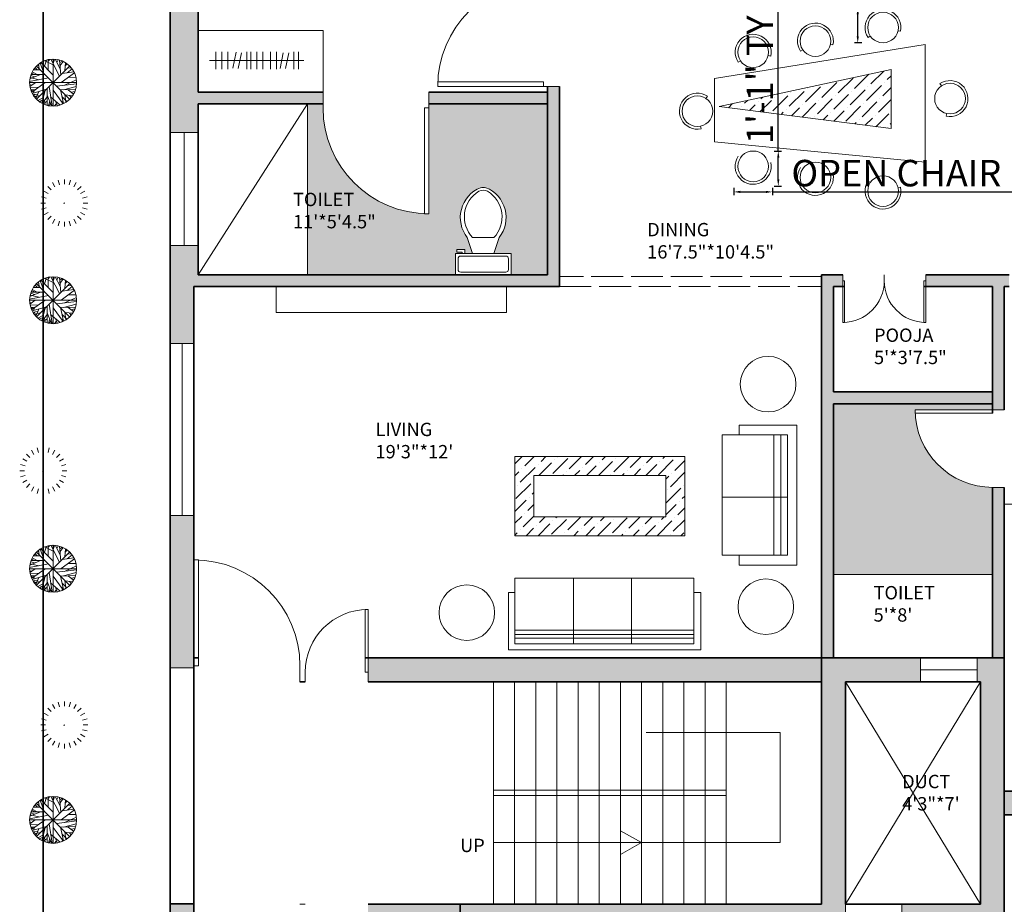
# Model space of a CAD drawing. Units: inches. Extents: x 2852 to 3654, y 1718 to 3031.
# Tile 3 of 5: x 2886 to 3257, y 2376 to 2711. Entities that reach past the tile are written whole.
import ezdxf

# ---------------------------------------------------------------- set-up
doc = ezdxf.new("R2010")
doc.units = ezdxf.units.IN
doc.linetypes.add('ACAD_ISO02W100', pattern=[15, 12, -3])
for name, color, linetype, lineweight in [('A-ANNO-DIMS', 2, 'Continuous', 18), ('A-ANNO-TEXT', 7, 'Continuous', 18), ('A-AREA-IDEN', 7, 'Continuous', 18), ('A-DOOR', 140, 'Continuous', 18), ('A-FLOR-CASE', 210, 'Continuous', 18), ('A-FLOR-FIXT', 9, 'Continuous', 18), ('A-FLOR-OPEN', 8, 'Continuous', 13), ('A-FLOR-PATT', 52, 'Continuous', 13), ('A-FLOR-STRS', 7, 'Continuous', 18), ('A-FURN-PATT', 210, 'Continuous', 13), ('A-WALL-OVHD', 140, 'ACAD_ISO02W100', 18), ('A-WALL-PATT', 12, 'Continuous', 13), ('C-PROP', 7, 'Continuous', 35), ('fur', 210, 'Continuous', 18), ('tree', 74, 'Continuous', 13), ('wall', 12, 'Continuous', 35), ('window', 140, 'Continuous', 18)]:
    doc.layers.add(name, color=color, linetype=linetype, lineweight=lineweight)
doc.styles.get("Standard").update_dxf_attribs({"font": 'arial.ttf'})
doc.dimstyles.new('ISO-25', dxfattribs={"dimtxt": 10, "dimasz": 2.5, "dimexe": 1.25, "dimexo": 0.625, "dimtad": 1, "dimdec": 0, "dimlunit": 4, "dimtxsty": 'Standard', "dimcen": 2.5, "dimadec": 0, "dimazin": 0, "dimtfac": 1, "dimtdec": 0, "dimtmove": 0, "dimatfit": 3, "dimfxl": 1, "dimarcsym": 0})

# ---------------------------------------------------------------- blocks, each defined once
blk = doc.blocks.new('*U2')
for p, q in [((0, 0), (0, -6)), ((40, 0), (40, -6))]:
    blk.add_line(p, q)
blk.add_lwpolyline([(0, 0), (0, 40), (1.75, 40), (1.75, 0)], close=True)
blk.add_arc((0, 0), 40, 0, 90)
blk = doc.blocks.new('*U4')
for p, q in [((9.5, -6), (9.5, -2)), ((-10, -8.5), (-8, -8.5)), ((-10, -9.5), (-10, -8.5)), ((-7, -9.5), (-10, -9.5)), ((-8, -8.5), (-8, -8)), ((-7, -8), (-7, -9.5)), ((-4, -8), (-6, -14)), ((4, -8), (6, -14)), ((4, -14), (-4, -14))]:
    blk.add_line(p, q)
blk.add_lwpolyline([(10.5, -8), (10.5, 0), (-10.5, 0), (-10.5, -8)], close=True)
for points in [[(-9.5, -2), (-9.5, -6)], [(8.5, -1), (-8.5, -1)], [(-8.5, -7), (8.5, -7)]]:
    blk.add_lwpolyline(points)
for centre, radius, start, end in [((-8.62, -1.88), 0.884, 81.8699, 188.1301), ((8.62, -1.88), 0.884, 351.8699, 98.1301), ((-8.62, -6.12), 0.884, 171.8699, 278.1301), ((8.62, -6.12), 0.884, 261.8699, 8.1301), ((3.52, -21.58), 12.17, 141.4691, 247.9714), ((4.2, -21.82), 11.33, 136.3677, 238.9468), ((-3.52, -21.58), 12.17, 292.0284, 38.5307), ((-4.2, -21.82), 11.33, 301.053, 43.6321), ((0, -27.88), 4, 245.7318, 294.2682), ((0, -29), 4, 254.8605, 285.1395)]:
    blk.add_arc(centre, radius, start, end)
blk = doc.blocks.new('*U10')
for p, q in [((-32.6092, 50.4264), (-23.2782, 23.5674)), ((-31.2008, 51.1035), (-0.2149, 20.1818)), ((-26.4472, 46.5894), (-26.2712, 53.8116)), ((-22.0458, 42.0753), (-16.5881, 57.6486)), ((-21.1656, 55.8436), (-0.0388, 45.0094)), ((-12.5388, 54.9406), (-7.9613, 59.4546)), ((-12.3627, 32.1443), (-12.5388, 58.7776)), ((-5.3205, 59.6806), (16.5105, 16.7963)), ((2.426, 54.9406), (-1.4472, 59.9056)), ((0, 59.9996), (0, -60)), ((0.4894, 48.6208), (3.6584, 59.6806)), ((18.2711, 35.5298), (5.419, 59.6806)), ((9.8203, 51.5549), (12.8133, 58.5516)), ((19.6795, 19.5047), (16.3344, 57.6486)), ((17.0387, 51.1035), (23.2006, 55.1666)), ((17.7429, 43.6552), (25.4894, 54.2636)), ((31.6513, 50.8778), (30.2429, 30.5643)), ((-53.2078, 27.4044), (-40.1797, 20.859)), ((-49.8627, 32.8214), (-32.7853, 32.8214)), ((-45.8134, 38.2383), (-40.5318, 33.0471)), ((-43.8768, 36.4326), (-44.405, 40.2696)), ((42, 42), (-42, -42)), ((42, -42), (-42, 42)), ((-40.1797, 44.558), (-36.4825, 43.2038)), ((-37.0107, 47.0408), (-35.25, 35.5298)), ((54.3626, 25.3731), (20.9119, 0.3198)), ((23.3767, 23.3417), (53.3063, 27.4044)), ((31.1232, 42.5267), (35.8767, 48.1693)), ((36.2288, 25.1474), (48.9049, 35.0784)), ((37.1091, 37.1098), (46.6161, 37.5612)), ((-59.7219, 2.8025), (-12.0106, 12.0565)), ((-32.2571, 20.6333), (-59.1937, 9.348)), ((-58.6656, 12.7336), (-35.9543, 7.5424)), ((-57.081, 17.9248), (-47.0458, 14.7649)), ((-56.0247, 20.859), (-20.8134, 20.859)), ((-54.7923, 24.4702), (-47.75, 21.0847)), ((-54.6162, -24.7335), (-20.2853, 0.0941)), ((29.3626, -6.6771), (59.4682, 7.091)), ((38.5175, 13.4107), (58.2359, 13.6364)), ((-60, 0), (60, 0)), ((-59.7219, -4.8714), (-54.2641, -6.6771)), ((-45.2853, -0.1316), (-59.0177, -10.0627)), ((-58.4895, -12.3197), (-36.4825, -11.6426)), ((-57.081, -18.4138), (-45.2853, -17.9624)), ((-52.6797, -18.188), (-55.4966, -22.0251)), ((-53.2078, -27.442), (-16.7641, -16.6081)), ((-47.2219, -19.3166), (-50.2148, -26.3135)), ((-35.9543, -22.4765), (-44.0529, -40.5329)), ((-19.9331, -20.2194), (-28.5599, -52.721)), ((-14.8275, -15.0282), (-14.6515, -57.6865)), ((-10.074, -10.0627), (-2.5036, -59.7178)), ((-0.0388, -19.0909), (25.8415, -53.8495)), ((9.2922, -9.1598), (59.6443, -2.8401)), ((18.6232, -18.6394), (26.7218, -53.3981)), ((18.7992, -18.6394), (57.3556, -17.2853)), ((26.3697, -18.4138), (58.9401, -9.8369)), ((38.1654, -18.188), (52.426, -29.0219)), ((45.9119, -24.0564), (55.595, -22.2508)), ((-38.9472, -29.0219), (-51.4472, -30.6018)), ((-46.5177, -30.1504), (-49.5106, -33.536)), ((-32.4331, -32.4075), (-48.1021, -35.5674)), ((-43.7008, -34.6645), (-46.6937, -37.373)), ((-24.6867, -37.8244), (-38.7712, -45.7241)), ((-26.2712, -43.9185), (-34.7219, -48.6583)), ((-14.6515, -36.2445), (-27.6797, -52.9467)), ((-14.6515, -47.3041), (-25.0388, -54.3009)), ((-21.5177, -45.4984), (-19.9331, -56.1065)), ((-14.6515, -32.1818), (-3.912, -59.4922)), ((-8.4895, -47.5298), (-11.4825, -58.5893)), ((-6.2008, -36.2445), (17.919, -57.0094)), ((5.9471, -46.6269), (10.5246, -58.5893)), ((22.8485, -36.4702), (35.3485, -48.4326)), ((24.7852, -44.8213), (23.0246, -54.978)), ((30.419, -30.1504), (32.3556, -50.0125)), ((31.4753, -31.279), (49.6091, -33.3103)), ((41.5105, -32.6332), (46.088, -38.0501)), ((-6.3768, -52.721), (-9.3698, -58.815)), ((8.4119, -53.1724), (3.8344, -59.4922))]:
    blk.add_line(p, q)
blk.add_circle((0, 0), 60)
blk = doc.blocks.new('*U9')
for p, q in [((-25.024, 42.079), (-31.077, 52.563)), ((-13.435, 46.72), (-16.606, 58.557)), ((-1.077, 60.601), (-1.077, 48.601)), ((11.28, 46.72), (14.452, 58.557)), ((22.87, 42.079), (28.923, 52.563)), ((-42.564, 24.554), (-53.039, 30.601)), ((-34.93, 34.454), (-43.503, 43.028)), ((32.776, 34.454), (41.349, 43.028)), ((40.409, 24.554), (50.884, 30.601)), ((-61.077, 0.601), (-49.077, 0.601)), ((-47.5, 13.04), (-59.033, 16.131)), ((45.346, 13.04), (56.878, 16.131)), ((58.923, 0.601), (46.923, 0.601)), ((-47.5, -11.837), (-59.033, -14.928)), ((-42.564, -23.351), (-53.039, -29.399)), ((40.409, -23.351), (50.884, -29.399)), ((45.346, -11.837), (56.878, -14.928)), ((-34.93, -33.251), (-43.503, -41.825)), ((-25.024, -40.876), (-31.077, -51.36)), ((-13.435, -45.517), (-16.606, -57.354)), ((-1.077, -59.399), (-1.077, -47.399)), ((11.28, -45.517), (14.452, -57.354)), ((22.87, -40.876), (28.923, -51.36)), ((32.776, -33.251), (41.349, -41.825))]:
    blk.add_line(p, q)
blk.add_lwpolyline([(-1.908, 0.978), (-2.67, -0.978), (0, 0)], close=True)
blk = doc.blocks.new('WARDROBE-HANGING-RAIL')
for p, q in [((2.45, 0), (2.45, 6.54)), ((4.63, 0), (4.63, 6.54)), ((6.93, 0), (6.93, 6.54)), ((8.87, 0.34), (10.08, 6.34)), ((10.83, 0.21), (12.05, 6.21)), ((14.06, 0), (14.06, 6.54)), ((15.59, 0), (15.59, 6.54)), ((17.86, 0), (17.86, 6.54)), ((20.11, 0), (20.11, 6.54)), ((23.04, 0), (23.04, 6.54)), ((25.39, 0), (25.39, 6.54)), ((26.68, 0.21), (27.9, 6.21)), ((28.71, 0.21), (29.93, 6.21)), ((31.85, 0), (31.85, 6.54)), ((33.7, 0), (33.7, 6.54)), ((0, 3.21), (35.71, 3.21))]:
    blk.add_line(p, q)
blk = doc.blocks.new('CHAIR-DINING-ROUND')
for p, q in [((12.45, 4.57), (13.43, 4.36)), ((1.15, 2.01), (1.98, 2.56))]:
    blk.add_line(p, q)
blk.add_circle((6.79, 5.79), 5.79)
blk.add_arc((6.79, 5.79), 6.79, 347.8419, 213.8526)
blk = doc.blocks.new('CHAIR-DINING-ROUND-OPEN')
blk.add_circle((6.79, 6.79), 5.79)
blk.add_arc((6.79, 6.79), 6.79, 146.1474, 12.1581)
blk = doc.blocks.new('*D29')
at = {"layer": 'A-ANNO-DIMS', "color": 0, "lineweight": -2, "transparency": 16777216}
for p, q in [((3204.28, 2715.63), (3204.28, 2718.45)), ((3206.78, 2717.2), (3216.43, 2717.2)), ((3218.93, 2715.63), (3218.93, 2718.45)), ((3218.93, 2717.2), (3408.86, 2717.2))]:
    blk.add_line(p, q, dxfattribs=at)
at = {"layer": 'A-ANNO-DIMS', "color": 0, "lineweight": 100, "transparency": 16777216}
for points in [[(3206.78, 2717.62), (3206.78, 2716.79), (3204.28, 2717.2)], [(3216.43, 2717.62), (3216.43, 2716.79), (3218.93, 2717.2)]]:
    blk.add_solid(points, dxfattribs=at)
at = {"layer": 'Defpoints', "color": 0, "lineweight": 100, "transparency": 16777216}
for p in [(3204.28, 2715.01), (3218.93, 2717.2), (3218.93, 2715.01)]:
    blk.add_point(p, dxfattribs=at)
at = {"layer": 'A-ANNO-DIMS', "color": 0, "transparency": 16777216, "insert": (3315.15, 2723), "char_height": 10, "attachment_point": 5}
blk.add_mtext('ROUND CHAIR 1\'-2 1/2" TYP.', dxfattribs=at)
blk = doc.blocks.new('*D30')
at = {"layer": 'A-ANNO-DIMS', "color": 0, "lineweight": -2, "transparency": 16777216}
for p, q in [((3202.08, 2715.01), (3202.08, 2778.77)), ((3203.66, 2715.01), (3200.83, 2715.01)), ((3202.08, 2704.26), (3202.08, 2712.51)), ((3203.66, 2701.76), (3200.83, 2701.76))]:
    blk.add_line(p, q, dxfattribs=at)
at = {"layer": 'A-ANNO-DIMS', "color": 0, "lineweight": 100, "transparency": 16777216}
for points in [[(3201.67, 2712.51), (3202.5, 2712.51), (3202.08, 2715.01)], [(3201.67, 2704.26), (3202.5, 2704.26), (3202.08, 2701.76)]]:
    blk.add_solid(points, dxfattribs=at)
at = {"layer": 'Defpoints', "color": 0, "lineweight": 100, "transparency": 16777216}
for p in [(3202.08, 2715.01), (3204.28, 2715.01), (3204.28, 2701.76)]:
    blk.add_point(p, dxfattribs=at)
at = {"layer": 'A-ANNO-DIMS', "color": 0, "transparency": 16777216, "insert": (3196.43, 2748.14), "char_height": 10, "attachment_point": 5, "rotation": 90}
blk.add_mtext('1\'-1" TYP.', dxfattribs=at)
blk = doc.blocks.new('*D31')
at = {"layer": 'A-ANNO-DIMS', "color": 0, "lineweight": -2, "transparency": 16777216}
for p, q in [((3155.23, 2647.04), (3155.23, 2644.22)), ((3157.73, 2645.47), (3167.38, 2645.47)), ((3169.88, 2647.04), (3169.88, 2644.22)), ((3169.88, 2645.47), (3348.61, 2645.47))]:
    blk.add_line(p, q, dxfattribs=at)
at = {"layer": 'A-ANNO-DIMS', "color": 0, "lineweight": 100, "transparency": 16777216}
for points in [[(3157.73, 2645.88), (3157.73, 2645.05), (3155.23, 2645.47)], [(3167.38, 2645.88), (3167.38, 2645.05), (3169.88, 2645.47)]]:
    blk.add_solid(points, dxfattribs=at)
at = {"layer": 'Defpoints', "color": 0, "lineweight": 100, "transparency": 16777216}
for p in [(3155.23, 2647.66), (3169.88, 2647.66), (3169.88, 2645.47)]:
    blk.add_point(p, dxfattribs=at)
at = {"layer": 'A-ANNO-DIMS', "color": 0, "transparency": 16777216, "insert": (3260.49, 2651.26), "char_height": 10, "attachment_point": 5}
blk.add_mtext('OPEN CHAIR 1\'-2 1/2" TYP.', dxfattribs=at)
blk = doc.blocks.new('*D32')
at = {"layer": 'A-ANNO-DIMS', "color": 0, "lineweight": -2, "transparency": 16777216}
for p, q in [((3172.08, 2660.9), (3172.08, 2724.67)), ((3170.5, 2660.9), (3173.33, 2660.9)), ((3172.08, 2650.16), (3172.08, 2658.4)), ((3170.5, 2647.66), (3173.33, 2647.66))]:
    blk.add_line(p, q, dxfattribs=at)
at = {"layer": 'A-ANNO-DIMS', "color": 0, "lineweight": 100, "transparency": 16777216}
for points in [[(3171.66, 2658.4), (3172.49, 2658.4), (3172.08, 2660.9)], [(3171.66, 2650.16), (3172.49, 2650.16), (3172.08, 2647.66)]]:
    blk.add_solid(points, dxfattribs=at)
at = {"layer": 'Defpoints', "color": 0, "lineweight": 100, "transparency": 16777216}
for p in [(3169.88, 2660.9), (3172.08, 2660.9), (3169.88, 2647.66)]:
    blk.add_point(p, dxfattribs=at)
at = {"layer": 'A-ANNO-DIMS', "color": 0, "transparency": 16777216, "insert": (3166.43, 2694.04), "char_height": 10, "attachment_point": 5, "rotation": 90}
blk.add_mtext('1\'-1" TYP.', dxfattribs=at)

msp = doc.modelspace()

# ---------------------------------------------------------------- hatches: boundary and pattern name
at = {"layer": 'A-FLOR-PATT'}
h = msp.add_hatch(dxfattribs=at)
h.set_pattern_fill('ANGLE', color=256)
h.set_pattern_definition([(0, (0, 0), (0, 6.985), [5.08, -1.905]), (90, (0, 0), (-6.985, 4e-16), [5.08, -1.905])])
h.paths.add_polyline_path([(3248.45, 2849.58), (3188.45, 2849.58), (3188.45, 2844.77), (3196.45, 2844.77), (3196.45, 2842.27), (3196.95, 2842.27), (3196.95, 2844.27), (3197.95, 2844.27), (3197.95, 2841.27), (3196.45, 2841.27), (3196.45, 2838.27), (3202.45, 2840.27, -0.501317), (3221.31, 2835.31, -0.132891), (3221.31, 2833.22, -0.501323), (3202.45, 2828.27), (3196.45, 2830.27), (3196.45, 2823.77), (3188.45, 2823.77), (3188.45, 2783.69), (3215.78, 2783.69), (3215.78, 2783.73, -0.401453), (3244.71, 2813.96), (3244.71, 2813.99), (3246.03, 2813.99), (3246.03, 2783.69), (3248.45, 2783.69)])
h.paths.add_polyline_path([(3420.95, 2714.69), (3324.42, 2714.69), (3324.42, 2691.18, -1), (3301.33, 2691.18), (3301.33, 2638.19), (3420.95, 2638.19)])
h.paths.add_polyline_path([(3059.57, 2647.05, -0.132891), (3061.66, 2647.05, -0.501323), (3066.62, 2628.19), (3064.62, 2622.19), (3071.12, 2622.19), (3071.12, 2614.19), (3084.95, 2614.19), (3084.95, 2678.69), (3040.14, 2678.69), (3040.14, 2677.19), (3040.14, 2637.19), (3038.39, 2637.19), (3038.39, 2637.23, -0.401453), (3000.14, 2677.19), (3000.14, 2678.69), (2994.25, 2678.69), (2994.25, 2614.19), (3050.12, 2614.19), (3050.12, 2622.19), (3052.62, 2622.19), (3052.62, 2622.69), (3050.62, 2622.69), (3050.62, 2623.69), (3053.62, 2623.69), (3053.62, 2622.19), (3056.62, 2622.19), (3054.62, 2628.19, -0.501317)])
h.paths.add_polyline_path([(3252.95, 2533.88, -0.400409), (3223.79, 2561.89), (3223.76, 2561.89), (3223.76, 2563.17), (3252.95, 2563.17), (3252.95, 2565.48), (3192.95, 2565.48), (3192.95, 2500.92), (3252.95, 2500.92)])
h.paths.add_polyline_path([(3248.45, 2338.72), (3188.45, 2338.72), (3188.45, 2271.48), (3248.45, 2271.48), (3248.45, 2273.69)])
h.paths.add_polyline_path([(3390.34, 2273.69), (3312.95, 2273.69), (3312.95, 2224.19), (3390.34, 2224.19)])
h.paths.add_polyline_path([(3365.33, 2231.19), (3382.33, 2231.19, -0.5), (3383.33, 2230.19), (3383.33, 2226.19, -0.5), (3382.33, 2225.19), (3365.33, 2225.19, -0.5), (3364.33, 2226.19), (3364.33, 2230.19, -0.5)], flags=16)
h.paths.add_polyline_path([(3372.19, 2255.72, -0.215004), (3375.48, 2255.72, -0.48008), (3377.83, 2238.19), (3369.83, 2238.19, -0.48008)], flags=16)
h.paths.add_polyline_path([(2987.37, 2220.07), (2951.37, 2220.07), (2951.37, 2095.57), (2987.37, 2095.57)])
at = {"layer": 'A-FURN-PATT'}
h = msp.add_hatch(dxfattribs=at)
h.set_pattern_fill('ANSI36', color=256)
h.paths.add_polyline_path([(3214.69, 2691.7), (3149.7, 2677.71), (3214.69, 2669.36)])
h = msp.add_hatch(dxfattribs=at)
h.set_pattern_fill('ANSI36', color=256)
h.paths.add_polyline_path([(3136.77, 2545.5), (3072.6, 2545.5), (3072.6, 2515.62), (3136.77, 2515.62)])
h.paths.add_polyline_path([(3079.75, 2538.36), (3129.62, 2538.36), (3129.62, 2522.76), (3079.75, 2522.76)], flags=16)
at = {"layer": 'A-WALL-PATT'}
h = msp.add_hatch(color=256, dxfattribs=at)
h.dxf.hatch_style = 1
h.paths.add_polyline_path([(2952.95, 2875.19), (2957.35, 2875.19), (2957.35, 2877.98), (2957.35, 2884.19), (2943.95, 2884.19), (2942.37, 2884.19), (2942.37, 2849.42), (2952.95, 2849.42)])
h.paths.add_polyline_path([(2952.95, 2706.39), (2952.95, 2749.45), (2942.37, 2749.45), (2942.37, 2667.89), (2952.95, 2667.89), (2952.95, 2678.69), (3000.14, 2678.69), (3000.14, 2683.19), (2952.95, 2683.19)])
h.paths.add_polyline_path([(2951.37, 2609.69), (3089.45, 2609.69), (3089.45, 2683.19), (3089.45, 2685.28), (3084.95, 2685.28), (3084.95, 2683.19), (3084.95, 2614.19), (2952.95, 2614.19), (2952.95, 2625.26), (2942.37, 2625.26), (2942.37, 2588.19), (2951.37, 2588.19)])
h.paths.add_polyline_path([(2951.37, 2506.48), (2951.37, 2523.26), (2942.37, 2523.26), (2942.37, 2465.69), (2951.37, 2465.69), (2951.37, 2466.48)])
h.paths.add_polyline_path([(2951.37, 2367.57), (2951.37, 2370.4), (2951.37, 2376.57), (2942.37, 2376.57), (2942.37, 2312.8), (2951.37, 2312.8), (2951.37, 2320.57), (2951.37, 2324.07)])
h.paths.add_polyline_path([(3051.87, 2324.07), (3047.37, 2324.07), (2951.37, 2324.07), (2951.37, 2320.57), (3047.37, 2320.57), (3047.37, 2296.57), (3047.37, 2266.82), (3051.87, 2266.82)])
h.paths.add_polyline_path([(2951.37, 2224.57), (2942.37, 2224.57), (2942.37, 2186.63), (2951.37, 2186.63), (2951.37, 2220.07)])
h.paths.add_polyline_path([(2951.37, 2247.87), (2942.37, 2247.87), (2942.37, 2224.57), (2951.37, 2224.57)])
h.paths.add_polyline_path([(3113.37, 2224.57), (2951.37, 2224.57), (2951.37, 2220.07), (3113.37, 2220.07)])
h.paths.add_polyline_path([(2951.37, 2121.7), (2942.37, 2121.7), (2942.37, 2086.57), (3113.37, 2086.57), (3147.16, 2086.57), (3147.16, 2095.57), (3113.37, 2095.57), (2951.37, 2095.57)])
h.paths.add_polyline_path([(3429.87, 2224.19), (3276.87, 2224.19), (3276.87, 2219.69), (3420.87, 2219.69), (3420.87, 2182.43), (3429.87, 2182.43)])
h.paths.add_polyline_path([(3276.87, 2175.85), (3272.37, 2175.85), (3272.37, 2095.57), (3240.86, 2095.57), (3240.86, 2086.57), (3276.87, 2086.57)])
h.paths.add_polyline_path([(3276.87, 2224.57), (3234.52, 2224.57), (3234.52, 2220.07), (3272.37, 2220.07), (3272.37, 2215.85), (3276.87, 2215.85)])
h = msp.add_hatch(color=256, dxfattribs=at)
h.dxf.hatch_style = 1
h.paths.add_polyline_path([(3188.45, 2469.48), (3017.1, 2469.48), (3017.1, 2464.04), (3017.1, 2460.48), (3188.45, 2460.48)])
h.paths.add_polyline_path([(3420.95, 2614.19), (3299.24, 2614.19), (3299.24, 2609.69), (3420.95, 2609.69)])
h.paths.add_polyline_path([(3429.95, 2614.19), (3420.95, 2614.19), (3420.95, 2609.69), (3420.95, 2543.19), (3429.95, 2543.19)])
h.paths.add_polyline_path([(3474.95, 2646.58), (3465.95, 2646.58), (3465.95, 2614.19), (3429.95, 2614.19), (3429.95, 2605.19), (3474.95, 2605.19)])
h.paths.add_polyline_path([(3474.95, 2747.69), (3429.95, 2747.69), (3429.95, 2791.96), (3420.95, 2791.96), (3420.95, 2743.19), (3420.95, 2738.69), (3425.23, 2738.69), (3465.95, 2738.69), (3465.95, 2711.51), (3474.95, 2711.51)])
h.paths.add_polyline_path([(3420.95, 2743.19), (3301.03, 2743.19), (3252.95, 2743.19), (3248.45, 2743.19), (3248.45, 2738.69), (3349.1, 2738.69), (3420.95, 2738.69)])
h.paths.add_polyline_path([(3188.92, 2779.19), (3179.45, 2779.19), (3179.45, 2747.69), (3165.97, 2747.69), (3165.97, 2742.11), (3165.97, 2738.69), (3188.92, 2738.69), (3212.98, 2738.69), (3212.98, 2743.19), (3188.92, 2743.19)])
h.paths.add_polyline_path([(3093.95, 2879.69), (3093.95, 2884.19), (3089.45, 2884.19), (3084.95, 2884.19), (3084.95, 2875.19), (3084.95, 2725.28), (3089.45, 2725.28), (3089.45, 2738.69), (3097.2, 2738.69), (3097.2, 2742.11), (3097.2, 2747.69), (3093.95, 2747.69)])
h.paths.add_polyline_path([(3188.45, 2875.19), (3202.27, 2875.19), (3202.27, 2884.19), (3179.45, 2884.19), (3179.45, 2879.69), (3179.45, 2779.19), (3188.92, 2779.19), (3215.78, 2779.19), (3215.78, 2783.69), (3188.45, 2783.69)])
h.paths.add_polyline_path([(3248.45, 2884.19), (3232.5, 2884.19), (3232.5, 2875.19), (3248.45, 2875.19)])
h.paths.add_polyline_path([(3252.95, 2875.19), (3248.45, 2875.19), (3248.45, 2778.22), (3252.95, 2778.22)])
h.paths.add_polyline_path([(3252.95, 2884.19), (3248.45, 2884.19), (3248.45, 2875.19), (3252.95, 2875.19)])
h.paths.add_polyline_path([(3259.75, 2884.19), (3252.95, 2884.19), (3252.95, 2875.19), (3259.75, 2875.19), (3259.75, 2877.98)])
h.paths.add_polyline_path([(3329.96, 2884.19), (3321.35, 2884.19), (3321.35, 2877.98), (3321.35, 2875.19), (3329.96, 2875.19)])
h.paths.add_polyline_path([(3029.12, 2884.19), (3018.95, 2884.19), (3018.95, 2877.98), (3018.95, 2875.19), (3029.12, 2875.19)])
h.paths.add_polyline_path([(3429.95, 2884.19), (3420.95, 2884.19), (3420.95, 2875.19), (3420.95, 2843.21), (3429.95, 2843.21)])
h = msp.add_hatch(color=256, dxfattribs=at)
h.dxf.hatch_style = 1
h.paths.add_polyline_path([(3084.95, 2683.19), (3040.14, 2683.19), (3040.14, 2678.69), (3084.95, 2678.69)])
h = msp.add_hatch(color=256, dxfattribs=at)
h.dxf.hatch_style = 1
h.paths.add_polyline_path([(3188.45, 2266.98), (3183.95, 2266.98), (3183.95, 2224.57), (3183.95, 2220.07), (3205.81, 2220.07), (3205.81, 2224.57), (3188.45, 2224.57)])
h.paths.add_polyline_path([(3188.45, 2367.48), (3183.95, 2367.48), (3183.95, 2266.98), (3188.45, 2266.98), (3188.45, 2271.48)])
h.paths.add_polyline_path([(3051.87, 2376.48), (3017.1, 2376.48), (3017.1, 2372.85), (3017.1, 2367.57), (3047.37, 2367.57), (3051.87, 2367.57), (3051.87, 2372.07)])
h.paths.add_polyline_path([(3197.45, 2376.48), (3197.45, 2460.48), (3225.82, 2460.48), (3225.82, 2469.48), (3188.45, 2469.48), (3188.45, 2376.48), (3051.87, 2376.48), (3051.87, 2372.07), (3051.87, 2367.48), (3197.45, 2367.48)])
h.paths.add_polyline_path([(3257.45, 2410.19), (3257.45, 2469.48), (3247.17, 2469.48), (3247.17, 2460.48), (3248.45, 2460.48), (3248.45, 2376.48), (3218.8, 2376.48), (3218.8, 2367.48), (3257.45, 2367.48)])
h.paths.add_polyline_path([(3257.45, 2367.48), (3252.95, 2367.48), (3252.95, 2278.19), (3257.45, 2278.19)])
h.paths.add_polyline_path([(3420.95, 2278.19), (3308.45, 2278.19), (3308.45, 2273.69), (3420.95, 2273.69)])
h.paths.add_polyline_path([(3257.45, 2527.51), (3257.45, 2533.88), (3252.95, 2533.88), (3252.95, 2469.48), (3257.45, 2469.48)])
h.paths.add_polyline_path([(3257.45, 2609.69), (3259.24, 2609.69), (3259.24, 2614.19), (3252.95, 2614.19), (3227.77, 2614.19), (3227.77, 2611.84), (3227.77, 2609.69), (3252.95, 2609.69), (3252.95, 2563.17), (3253.06, 2563.17), (3257.45, 2563.17)])
h.paths.add_polyline_path([(3196.43, 2614.19), (3188.45, 2614.19), (3188.45, 2569.84), (3188.45, 2469.48), (3192.95, 2469.48), (3192.95, 2565.48), (3252.95, 2565.48), (3252.95, 2569.98), (3192.95, 2569.98), (3192.95, 2609.69), (3196.43, 2609.69), (3196.43, 2611.84)])
h = msp.add_hatch(color=256, dxfattribs=at)
h.dxf.hatch_style = 1
h.paths.add_polyline_path([(3429.87, 2117.5), (3420.87, 2117.5), (3420.87, 2095.19), (3276.87, 2095.19), (3276.87, 2086.19), (3429.87, 2086.19)])
h.paths.add_polyline_path([(3429.95, 2278.19), (3420.95, 2278.19), (3420.95, 2273.69), (3420.95, 2224.19), (3429.95, 2224.19)])
h.paths.add_polyline_path([(3429.95, 2309.24), (3420.95, 2309.24), (3420.95, 2278.19), (3429.95, 2278.19)])
h.paths.add_polyline_path([(3429.95, 2419.19), (3420.95, 2419.19), (3420.95, 2410.19), (3420.95, 2374.17), (3429.95, 2374.17)])
h.paths.add_polyline_path([(3429.95, 2478.26), (3420.95, 2478.26), (3420.95, 2419.19), (3429.95, 2419.19)])
h.paths.add_polyline_path([(3420.95, 2419.19), (3257.45, 2419.19), (3257.45, 2410.19), (3283.32, 2410.19), (3420.95, 2410.19)])

# ---------------------------------------------------------------- linework, layer by layer
at = {"layer": 'A-FLOR-CASE'}
for points in [[(3000.14, 2683.19), (2952.95, 2683.19), (2952.95, 2706.39), (3000.14, 2706.39)], [(2982.4, 2609.69), (3069.46, 2609.69), (3069.46, 2599.92), (2982.4, 2599.92)], [(3257.45, 2419.19), (3283.32, 2419.19), (3283.32, 2527.51), (3257.45, 2527.51)]]:
    msp.add_lwpolyline(points, close=True, dxfattribs=at)
at = {"layer": 'A-FLOR-FIXT'}
for p, q in [((2994.25, 2678.69), (2952.95, 2614.19)), ((2994.25, 2678.69), (2994.25, 2614.19)), ((2994.25, 2614.19), (2994.25, 2678.69)), ((3192.95, 2500.92), (3252.95, 2500.92))]:
    msp.add_line(p, q, dxfattribs=at)
at = {"layer": 'A-FLOR-OPEN'}
for p, q in [((3197.45, 2376.48), (3248.45, 2460.48)), ((3197.45, 2460.48), (3248.45, 2376.48))]:
    msp.add_line(p, q, dxfattribs=at)
at = {"layer": 'A-FLOR-STRS'}
for p, q in [((3064.45, 2460.48), (3064.45, 2376.48)), ((3072.45, 2460.48), (3072.45, 2376.48)), ((3080.45, 2460.48), (3080.45, 2376.48)), ((3088.45, 2460.48), (3088.45, 2376.48)), ((3096.45, 2460.48), (3096.45, 2376.48)), ((3104.45, 2460.48), (3104.45, 2376.48)), ((3112.45, 2460.48), (3112.45, 2376.48)), ((3120.45, 2460.48), (3120.45, 2376.48)), ((3128.45, 2460.48), (3128.45, 2376.48)), ((3136.45, 2460.48), (3136.45, 2376.48)), ((3144.45, 2460.48), (3144.45, 2376.48)), ((3188.45, 2460.48), (3152.45, 2460.48)), ((3152.45, 2460.48), (3152.45, 2376.48)), ((3172.75, 2441.31), (3122.2, 2441.31)), ((3172.75, 2399.69), (3172.75, 2441.31)), ((3073.18, 2419.48), (3064.45, 2419.48)), ((3073.18, 2417.48), (3064.45, 2417.48)), ((3152.45, 2419.48), (3073.18, 2419.48)), ((3152.45, 2417.48), (3073.18, 2417.48)), ((3120.45, 2399.69), (3112.45, 2404.14)), ((3064.45, 2399.69), (3172.75, 2399.69)), ((3120.45, 2399.69), (3112.45, 2395.23))]:
    msp.add_line(p, q, dxfattribs=at)
at = {"layer": 'A-WALL-OVHD'}
msp.add_line((2991.37, 2376.4), (2993.37, 2376.4), dxfattribs=at)
msp.add_lwpolyline([(3089.45, 2609.69), (3188.45, 2609.69), (3188.45, 2613.48), (3089.45, 2613.48)], close=True, dxfattribs=at)
at = {"layer": 'C-PROP'}
msp.add_line((2894.37, 1890.07), (2894.37, 2927.69), dxfattribs=at)
at = {"layer": 'fur'}
for p, q in [((3148.02, 2688.25), (3227.51, 2701.18)), ((3227.51, 2701.18), (3227.51, 2656.66)), ((3214.69, 2691.7), (3149.7, 2677.71)), ((3214.69, 2669.36), (3214.69, 2691.7)), ((3148.02, 2664.36), (3148.02, 2688.25)), ((3149.7, 2677.71), (3214.69, 2669.36)), ((3160.83, 2663.08), (3148.02, 2664.36)), ((3227.51, 2656.66), (3160.83, 2663.08)), ((3157.25, 2553.73), (3157.25, 2557.35)), ((3157.25, 2557.35), (3179.11, 2557.35)), ((3179.11, 2557.35), (3179.11, 2504.52)), ((3170.45, 2553.73), (3170.45, 2508.24)), ((3173.08, 2553.73), (3173.08, 2508.24)), ((3175.61, 2553.73), (3175.61, 2508.24)), ((3175.61, 2530.15), (3150.91, 2530.15)), ((3175.61, 2508.24), (3150.91, 2508.24)), ((3157.25, 2504.52), (3157.25, 2508.24)), ((3179.11, 2504.52), (3157.25, 2504.52)), ((3094.73, 2474.83), (3094.73, 2499.53)), ((3116.64, 2474.83), (3116.64, 2499.53)), ((3072.59, 2494.12), (3070.13, 2494.12)), ((3070.13, 2494.12), (3070.13, 2472.55)), ((3142.84, 2494.12), (3140.22, 2494.12)), ((3142.84, 2472.55), (3142.84, 2494.12)), ((3072.59, 2479.88), (3140.22, 2479.88)), ((3072.59, 2478.36), (3140.22, 2478.36)), ((3072.59, 2476.88), (3140.22, 2476.88)), ((3070.13, 2472.55), (3142.84, 2472.55))]:
    msp.add_line(p, q, dxfattribs=at)
msp.add_lwpolyline([(3175.61, 2508.24), (3175.61, 2553.73), (3150.91, 2553.73), (3150.91, 2508.24)], dxfattribs=at)
for points in [[(3072.6, 2515.62), (3136.77, 2515.62), (3136.77, 2545.5), (3072.6, 2545.5)], [(3079.75, 2522.76), (3129.62, 2522.76), (3129.62, 2538.36), (3079.75, 2538.36)], [(3072.59, 2474.83), (3140.22, 2474.83), (3140.22, 2499.53), (3072.59, 2499.53)]]:
    msp.add_lwpolyline(points, close=True, dxfattribs=at)
for centre in [(3168.23, 2572.85), (3167.38, 2488.79), (3054.42, 2486.56)]:
    msp.add_circle(centre, 10.5, dxfattribs=at)
at = {"layer": 'wall'}
for p, q in [((2942.37, 2224.57), (2942.37, 2884.19)), ((2952.95, 2683.19), (2952.95, 2875.19)), ((3084.95, 2685.28), (3084.95, 2683.19)), ((3089.45, 2685.28), (3089.45, 2678.69)), ((3000.14, 2683.19), (2952.95, 2683.19)), ((3084.95, 2683.19), (3040.14, 2683.19)), ((3084.95, 2614.19), (3084.95, 2683.19)), ((3089.45, 2609.69), (3089.45, 2683.19)), ((2952.95, 2678.69), (2952.95, 2614.19)), ((2952.95, 2678.69), (3000.14, 2678.69)), ((3040.14, 2678.69), (3084.95, 2678.69)), ((2952.95, 2614.19), (3084.95, 2614.19)), ((3188.45, 2569.84), (3188.45, 2614.19)), ((3196.43, 2614.19), (3188.45, 2614.19)), ((3188.45, 2569.98), (3188.45, 2613.48)), ((3188.45, 2613.48), (3188.45, 2604.88)), ((3252.95, 2614.19), (3227.77, 2614.19)), ((3259.24, 2614.19), (3252.95, 2614.19)), ((2951.37, 2609.69), (3089.45, 2609.69)), ((2951.37, 2609.69), (2951.37, 2367.57)), ((2951.37, 2609.69), (2951.37, 2465.69)), ((3192.95, 2569.98), (3192.95, 2609.69)), ((3197.12, 2609.69), (3192.95, 2609.69)), ((3212.25, 2609.69), (3211.95, 2609.69)), ((3252.95, 2609.69), (3227.08, 2609.69)), ((3252.95, 2561.89), (3252.95, 2609.69)), ((3259.24, 2609.69), (3257.45, 2609.69)), ((3257.45, 2563.17), (3257.45, 2609.69)), ((3252.95, 2569.98), (3192.95, 2569.98)), ((3188.45, 2469.48), (3188.45, 2569.84)), ((3252.95, 2565.48), (3192.95, 2565.48)), ((3192.95, 2469.48), (3192.95, 2565.48)), ((3252.95, 2561.89), (3252.95, 2565.48)), ((3252.95, 2469.48), (3252.95, 2533.88)), ((3252.95, 2469.48), (3252.95, 2533.88)), ((3257.45, 2469.48), (3257.45, 2533.88)), ((2951.37, 2469.48), (2953.12, 2469.48)), ((3016.06, 2469.48), (3188.45, 2469.48)), ((3188.45, 2469.48), (3188.45, 2376.48)), ((3257.45, 2469.48), (3188.45, 2469.48)), ((3257.45, 2367.48), (3257.45, 2469.48)), ((2991.37, 2460.48), (2993.37, 2460.48)), ((3017.1, 2460.48), (3188.45, 2460.48)), ((3248.45, 2460.48), (3197.45, 2460.48)), ((3197.45, 2460.48), (3197.45, 2376.48)), ((3248.45, 2376.48), (3248.45, 2460.48)), ((3248.45, 2419.19), (3248.45, 2376.48)), ((3429.95, 2419.19), (3257.45, 2419.19)), ((3420.95, 2410.19), (3257.45, 2410.19)), ((2943.37, 2376.57), (2942.37, 2376.57)), ((2943.37, 2376.57), (2951.37, 2376.57)), ((3051.87, 2376.48), (3017.1, 2376.48)), ((3051.87, 2376.48), (3188.45, 2376.48)), ((3051.87, 2372.07), (3051.87, 2376.48)), ((3197.45, 2376.48), (3248.45, 2376.48))]:
    msp.add_line(p, q, dxfattribs=at)
at = {"layer": 'window'}
for p, q in [((2947.66, 2625.26), (2947.66, 2667.89)), ((2946.87, 2523.26), (2946.87, 2588.19)), ((3225.82, 2464.98), (3247.17, 2464.98))]:
    msp.add_line(p, q, dxfattribs=at)
for points in [[(2942.37, 2667.89), (2952.95, 2667.89), (2952.95, 2625.26), (2942.37, 2625.26)], [(2942.37, 2588.19), (2951.37, 2588.19), (2951.37, 2523.26), (2942.37, 2523.26)], [(3225.82, 2469.48), (3247.17, 2469.48), (3247.17, 2460.48), (3225.82, 2460.48)], [(2951.37, 2465.69), (2942.37, 2465.69), (2942.37, 2376.57), (2951.37, 2376.57)], [(3197.45, 2376.48), (3218.8, 2376.48), (3218.8, 2367.48), (3197.45, 2367.48)]]:
    msp.add_lwpolyline(points, close=True, dxfattribs=at)

# ---------------------------------------------------------------- block references
at = {"layer": 'A-DOOR'}
for p, rotation in [((3083.45, 2685.28), 90), ((3040.14, 2677.19), 180)]:
    msp.add_blockref('*U2', p, dxfattribs=dict(at, rotation=rotation))
for p, xscale, yscale, zscale, rotation in [((3196.43, 2611.84), -0.3917212815103202, 0.3917212815103202, 0.3917212815103202, 180), ((3227.77, 2611.84), 0.3917212815103202, 0.3917212815103202, 0.3917212815103202, 180), ((3253.06, 2563.17), -0.7324393954917942, 0.7324393954917942, 0.7324393954917942, 90)]:
    msp.add_blockref('*U2', p, dxfattribs=dict(at, xscale=xscale, yscale=yscale, zscale=zscale, rotation=rotation))
msp.add_blockref('*U2', (2951.37, 2466.48), dxfattribs=at)
at = {"layer": 'A-DOOR', "xscale": -0.5931757633417637, "yscale": 0.5931757633417637, "zscale": 0.5931757633417637}
msp.add_blockref('*U2', (3017.1, 2464.04), dxfattribs=at)
at = {"layer": 'A-FLOR-CASE'}
msp.add_blockref('WARDROBE-HANGING-RAIL', (2957.21, 2691.84), dxfattribs=at)
at = {"layer": 'A-FLOR-FIXT', "xscale": -1, "rotation": 180}
msp.add_blockref('*U4', (3060.62, 2614.19), dxfattribs=at)
at = {"layer": 'fur'}
for name, p in [('CHAIR-DINING-ROUND', (3204.85, 2701.76)), ('CHAIR-DINING-ROUND', (3179.31, 2696.62)), ('CHAIR-DINING-ROUND', (3155.8, 2692.43)), ('CHAIR-DINING-ROUND-OPEN', (3155.8, 2648.33)), ('CHAIR-DINING-ROUND-OPEN', (3179.31, 2644.14))]:
    msp.add_blockref(name, p, dxfattribs=at)
for p, rotation in [((3231.15, 2687.5), 270.0000000000006), ((3144.4, 2667.51), 68.30546771060055), ((3220.09, 2648.65), 158.3054677105967)]:
    msp.add_blockref('CHAIR-DINING-ROUND', p, dxfattribs=dict(at, rotation=rotation))
at = {"layer": 'tree', "xscale": 0.1480989313836924, "yscale": 0.1480989313836924, "zscale": 0.1480989313836924}
for name, p in [('*U10', (2898.14, 2686.73)), ('*U9', (2902.57, 2641.18)), ('*U10', (2898.14, 2604.55)), ('*U9', (2894.58, 2540.08)), ('*U10', (2898.14, 2503.15)), ('*U9', (2902.57, 2444.07)), ('*U10', (2898.14, 2408.29))]:
    msp.add_blockref(name, p, dxfattribs=at)

# ---------------------------------------------------------------- texts
at = {"layer": 'A-ANNO-TEXT', "insert": (3051.89, 2401.17), "char_height": 5.041, "attachment_point": 1}
msp.add_mtext_dynamic_manual_height_columns('UP', width=98.3816, gutter_width=25.21, heights=[0], dxfattribs=at)
at = {"layer": 'A-AREA-IDEN', "attachment_point": 1}
for s, insert, char_height in [('TOILET\\P11\'*5\'4.5"', (2988.76, 2645.14), 5.041), ('DINING\\P16\'7.5"*10\'4.5"', (3122.57, 2633.74), 5.0412), ('POOJA\\P5\'*3\'7.5"', (3208.24, 2593.87), 5.041), ('LIVING\\P19\'3"*12\'', (3019.94, 2558.28), 5.041), ("TOILET\\P5'*8'", (3208.07, 2496.61), 5.041), ('DUCT\\P4\'3"*7\'', (3218.86, 2425.3), 5.041)]:
    msp.add_mtext_dynamic_manual_height_columns(s, width=98.3816, gutter_width=25.21, heights=[0], dxfattribs=dict(at, insert=insert, char_height=char_height))

# ---------------------------------------------------------------- dimensions: what is measured, and where the dimension line sits
at = {"layer": 'A-ANNO-DIMS'}
for base, p1, p2, picture, middle in [((3202.0837, 2715.0052), (3204.2806, 2701.7636), (3204.2806, 2715.0052), '*D30', (3196.4349, 2748.1371)), ((3172.08, 2660.9), (3169.88, 2647.66), (3169.88, 2660.9), '*D32', (3166.43, 2694.04))]:
    dim = msp.add_linear_dim(base=base, p1=p1, p2=p2, angle=90, text='<> TYP.', dimstyle='ISO-25', override={"dimdec": 1, "dimlfac": 1, "dimrnd": 0, "dimzin": 1, "dimdsep": 46, "dimlunit": 4, "dimfrac": 2}, dxfattribs=at)
    dim.commit()
    dim.dimension.update_dxf_attribs({"geometry": picture, "text_midpoint": middle})
for base, p1, p2, text, picture, middle in [((3218.9266, 2717.2021), (3204.2806, 2715.0052), (3218.9266, 2715.0052), 'ROUND CHAIR <> TYP.', '*D29', (3315.145, 2723.0011)), ((3169.8784, 2645.4653), (3155.2325, 2647.6622), (3169.8784, 2647.6622), 'OPEN CHAIR <> TYP.', '*D31', (3260.4932, 2651.2642))]:
    dim = msp.add_linear_dim(base=base, p1=p1, p2=p2, text=text, dimstyle='ISO-25', override={"dimdec": 1, "dimlfac": 1, "dimrnd": 0, "dimzin": 1, "dimdsep": 46, "dimlunit": 4, "dimfrac": 2}, dxfattribs=at)
    dim.commit()
    dim.dimension.update_dxf_attribs({"geometry": picture, "text_midpoint": middle})

doc.saveas('drawing.dxf')
